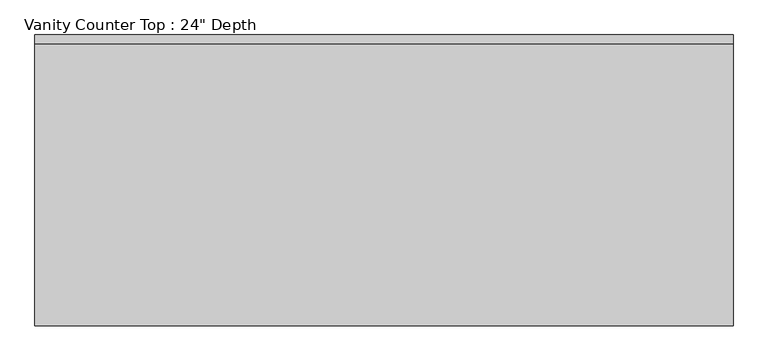
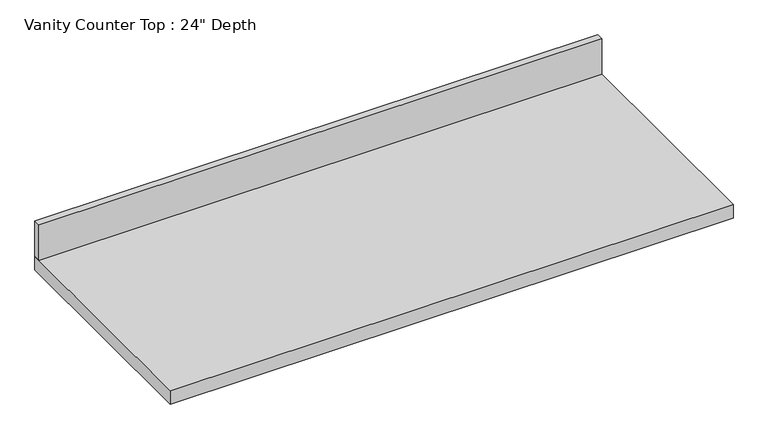
"""IFC4 building model written with IfcOpenShell, lengths in millimetres: furniture geometry."""

from ifc_helpers import new_model, si_unit, frame, origin, place, context, project, spatial, polyline, outline, extrude, source, transform, mapped, element, save


def furniture_32cec9f0(model_context):
    return source(origin(), model_context, "Body", "SweptSolid", [
        extrude(outline(polyline([(323.5377049, 0.0), (323.5377049, -635.0), (-1200.4622951, -635.0), (-1200.4622951, 0.0), (323.5377049, 0.0)])), frame((0.0, 0.0, 749.3), z_axis=(0.0, 0.0, 1.0), x_axis=(1.0, 0.0, 0.0)), (0.0, 0.0, 1.0), 38.1),
        extrude(outline(polyline([(-1200.4622951, 0.0), (323.5377049, 0.0), (323.5377049, -19.05), (-1200.4622951, -19.05), (-1200.4622951, 0.0)])), frame((0.0, 0.0, 787.4), z_axis=(0.0, 0.0, 1.0), x_axis=(1.0, 0.0, 0.0)), (0.0, 0.0, 1.0), 101.6),
    ])


if __name__ == "__main__":
    model = new_model("IFC4")
    model_context = context("Model", 3, world=origin())
    ifc_project = project(units=[si_unit("LENGTHUNIT", "METRE", prefix="MILLI")], contexts=[model_context])
    site = spatial("IfcSite", under=ifc_project)
    building = spatial("IfcBuilding", under=site)
    placement = place(None, origin())
    furniture_shape = furniture_32cec9f0(model_context)
    element("IfcFurniture", 1, ObjectType="Vanity Counter Top : 24\" Depth", at=placement, inside=building, context=model_context, shape_type="MappedRepresentation", body=[
        mapped(furniture_shape, transform((0.0, 0.0, 0.0), x_axis=(1.0, 0.0, 0.0), y_axis=(0.0, 1.0, 0.0), z_axis=(0.0, 0.0, 1.0))),
    ])
    save(model, "model.ifc")

# Revit data of these elements
# Type "Vanity Counter Top : 24\" Depth"
#   Counter Thickness = 0' - 1 1/2"
#   Depth = 2' - 1"
#   Height = 2' - 7"
#   Length [instance default] = 4' - 0"
#   Counter Top Material = Counter Top
#   Default Elevation = 0
# Element 1 (IfcFurniture, "Vanity Counter Top : 24\" Depth")
#   Length = 5' - 0"
#   Materials on its faces: "Counter Top"
# Materials
#   "Counter Top": class "Wood", colour RGB 226 177 128, transparency 0
